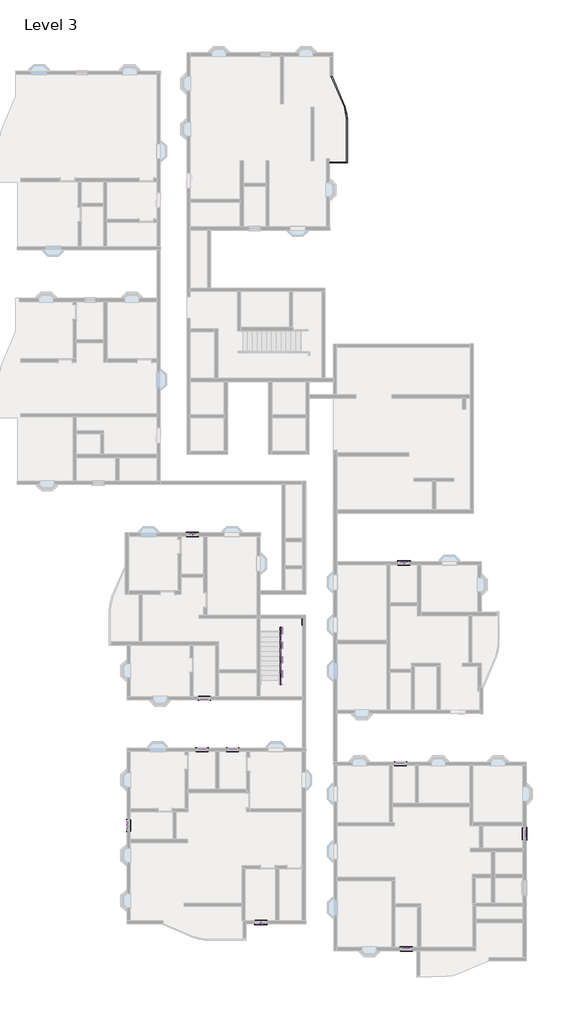
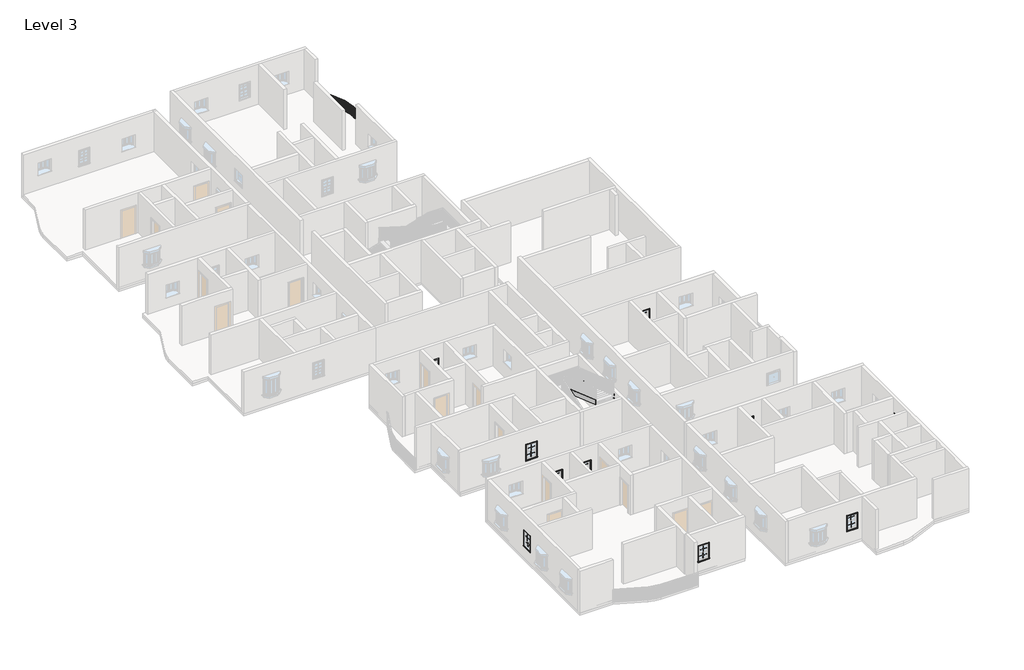
# One storey, part 13 of 14: 40 proxies, 6 members, 1 railing.
"""IFC4 building model written with IfcOpenShell, lengths in millimetres."""

from ifc_helpers import new_model, si_unit, frame, origin, place, context, project, spatial, polyline, circle_curve, outline, extrude, transform, mapped, element, save
from ifc_brep_helpers import plane_surface, cylinder_surface, revolved_surface, advanced_brep
from components import muntin_pattern_2x2_muntin_pattern_2x2_c35c595f, trim_window_exterior_flat_with_sill_e38017c9, trim_window_interior_flat_picture_frame_d728ed12

model = new_model("IFC4")

# Units and contexts
model_context = context("Model", 3, world=origin())
ifc_project = project(units=[si_unit("LENGTHUNIT", "METRE", prefix="MILLI")], contexts=[model_context])

# Site, building, storey
site = spatial("IfcSite", under=ifc_project)
building = spatial("IfcBuilding", under=site)
storey = spatial("IfcBuildingStorey", under=building, Name="Level 3", Elevation=6096.0)

# Proxies
placement = place(None, origin())
muntin_pattern_2x2_muntin_pattern_2x2_shape = muntin_pattern_2x2_muntin_pattern_2x2_c35c595f(model_context)
element("IfcBuildingElementProxy", 1, Name="Muntin Pattern_2x2 : Muntin Pattern_2x2", ObjectType="Muntin Pattern_2x2 : Muntin Pattern_2x2", at=placement, inside=storey, context=model_context, shape_type="MappedRepresentation", body=[
    mapped(muntin_pattern_2x2_muntin_pattern_2x2_shape, transform((-8150.287215, -357.5666506, 7566.025), x_axis=(1.0, 0.0, 0.0), y_axis=(0.0, 1.0, 0.0), z_axis=(0.0, 0.0, 1.0))),
])
element("IfcBuildingElementProxy", 2, Name="Muntin Pattern_2x2 : Muntin Pattern_2x2", ObjectType="Muntin Pattern_2x2 : Muntin Pattern_2x2", at=placement, inside=storey, context=model_context, shape_type="MappedRepresentation", body=[
    mapped(muntin_pattern_2x2_muntin_pattern_2x2_shape, transform((-8150.287215, -402.0166506, 7086.6), x_axis=(1.0, 0.0, 0.0), y_axis=(0.0, 1.0, 0.0), z_axis=(0.0, 0.0, 1.0))),
])
element("IfcBuildingElementProxy", 3, Name="Muntin Pattern_2x2 : Muntin Pattern_2x2", ObjectType="Muntin Pattern_2x2 : Muntin Pattern_2x2", at=placement, inside=storey, context=model_context, shape_type="MappedRepresentation", body=[
    mapped(muntin_pattern_2x2_muntin_pattern_2x2_shape, transform((-7397.812215, -10854.1166506, 7566.025), x_axis=(-1.0, 0.0, 0.0), y_axis=(0.0, -1.0, 0.0), z_axis=(0.0, 0.0, 1.0))),
])
element("IfcBuildingElementProxy", 4, Name="Muntin Pattern_2x2 : Muntin Pattern_2x2", ObjectType="Muntin Pattern_2x2 : Muntin Pattern_2x2", at=placement, inside=storey, context=model_context, shape_type="MappedRepresentation", body=[
    mapped(muntin_pattern_2x2_muntin_pattern_2x2_shape, transform((-7397.812215, -10809.6666506, 7086.6), x_axis=(-1.0, 0.0, 0.0), y_axis=(0.0, -1.0, 0.0), z_axis=(0.0, 0.0, 1.0))),
])
element("IfcBuildingElementProxy", 5, Name="Muntin Pattern_2x2 : Muntin Pattern_2x2", ObjectType="Muntin Pattern_2x2 : Muntin Pattern_2x2", at=placement, inside=storey, context=model_context, shape_type="MappedRepresentation", body=[
    mapped(muntin_pattern_2x2_muntin_pattern_2x2_shape, transform((-7540.687215, -13997.3666506, 7566.025), x_axis=(1.0, 0.0, 0.0), y_axis=(0.0, 1.0, 0.0), z_axis=(0.0, 0.0, 1.0))),
])
element("IfcBuildingElementProxy", 6, Name="Muntin Pattern_2x2 : Muntin Pattern_2x2", ObjectType="Muntin Pattern_2x2 : Muntin Pattern_2x2", at=placement, inside=storey, context=model_context, shape_type="MappedRepresentation", body=[
    mapped(muntin_pattern_2x2_muntin_pattern_2x2_shape, transform((-7540.687215, -14041.8166506, 7086.6), x_axis=(1.0, 0.0, 0.0), y_axis=(0.0, 1.0, 0.0), z_axis=(0.0, 0.0, 1.0))),
])
element("IfcBuildingElementProxy", 7, Name="Muntin Pattern_2x2 : Muntin Pattern_2x2", ObjectType="Muntin Pattern_2x2 : Muntin Pattern_2x2", at=placement, inside=storey, context=model_context, shape_type="MappedRepresentation", body=[
    mapped(muntin_pattern_2x2_muntin_pattern_2x2_shape, transform((-5597.587215, -13997.3666506, 7566.025), x_axis=(1.0, 0.0, 0.0), y_axis=(0.0, 1.0, 0.0), z_axis=(0.0, 0.0, 1.0))),
])
element("IfcBuildingElementProxy", 8, Name="Muntin Pattern_2x2 : Muntin Pattern_2x2", ObjectType="Muntin Pattern_2x2 : Muntin Pattern_2x2", at=placement, inside=storey, context=model_context, shape_type="MappedRepresentation", body=[
    mapped(muntin_pattern_2x2_muntin_pattern_2x2_shape, transform((-5597.587215, -14041.8166506, 7086.6), x_axis=(1.0, 0.0, 0.0), y_axis=(0.0, 1.0, 0.0), z_axis=(0.0, 0.0, 1.0))),
])
element("IfcBuildingElementProxy", 9, Name="Muntin Pattern_2x2 : Muntin Pattern_2x2", ObjectType="Muntin Pattern_2x2 : Muntin Pattern_2x2", at=placement, inside=storey, context=model_context, shape_type="MappedRepresentation", body=[
    mapped(muntin_pattern_2x2_muntin_pattern_2x2_shape, transform((-12255.562215, -18863.6994419, 7566.025), x_axis=(0.0, 1.0, 0.0), y_axis=(-1.0, 0.0, 0.0), z_axis=(0.0, 0.0, 1.0))),
])
element("IfcBuildingElementProxy", 10, Name="Muntin Pattern_2x2 : Muntin Pattern_2x2", ObjectType="Muntin Pattern_2x2 : Muntin Pattern_2x2", at=placement, inside=storey, context=model_context, shape_type="MappedRepresentation", body=[
    mapped(muntin_pattern_2x2_muntin_pattern_2x2_shape, transform((-12211.112215, -18863.6994419, 7086.6), x_axis=(0.0, 1.0, 0.0), y_axis=(-1.0, 0.0, 0.0), z_axis=(0.0, 0.0, 1.0))),
])
element("IfcBuildingElementProxy", 11, Name="Muntin Pattern_2x2 : Muntin Pattern_2x2", ObjectType="Muntin Pattern_2x2 : Muntin Pattern_2x2", at=placement, inside=storey, context=model_context, shape_type="MappedRepresentation", body=[
    mapped(muntin_pattern_2x2_muntin_pattern_2x2_shape, transform((-3806.2891351, -25065.4166506, 7566.025), x_axis=(-1.0, 0.0, 0.0), y_axis=(0.0, -1.0, 0.0), z_axis=(0.0, 0.0, 1.0))),
])
element("IfcBuildingElementProxy", 12, Name="Muntin Pattern_2x2 : Muntin Pattern_2x2", ObjectType="Muntin Pattern_2x2 : Muntin Pattern_2x2", at=placement, inside=storey, context=model_context, shape_type="MappedRepresentation", body=[
    mapped(muntin_pattern_2x2_muntin_pattern_2x2_shape, transform((-3806.2891351, -25020.9666506, 7086.6), x_axis=(-1.0, 0.0, 0.0), y_axis=(0.0, -1.0, 0.0), z_axis=(0.0, 0.0, 1.0))),
])
element("IfcBuildingElementProxy", 13, Name="Muntin Pattern_2x2 : Muntin Pattern_2x2", ObjectType="Muntin Pattern_2x2 : Muntin Pattern_2x2", at=placement, inside=storey, context=model_context, shape_type="MappedRepresentation", body=[
    mapped(muntin_pattern_2x2_muntin_pattern_2x2_shape, transform((5410.0380523, -26615.6292694, 7566.025), x_axis=(1.0, 0.0, 0.0), y_axis=(0.0, 1.0, 0.0), z_axis=(0.0, 0.0, 1.0))),
])
element("IfcBuildingElementProxy", 14, Name="Muntin Pattern_2x2 : Muntin Pattern_2x2", ObjectType="Muntin Pattern_2x2 : Muntin Pattern_2x2", at=placement, inside=storey, context=model_context, shape_type="MappedRepresentation", body=[
    mapped(muntin_pattern_2x2_muntin_pattern_2x2_shape, transform((5410.0380523, -26660.0792694, 7086.6), x_axis=(1.0, 0.0, 0.0), y_axis=(0.0, 1.0, 0.0), z_axis=(0.0, 0.0, 1.0))),
])
element("IfcBuildingElementProxy", 15, Name="Muntin Pattern_2x2 : Muntin Pattern_2x2", ObjectType="Muntin Pattern_2x2 : Muntin Pattern_2x2", at=placement, inside=storey, context=model_context, shape_type="MappedRepresentation", body=[
    mapped(muntin_pattern_2x2_muntin_pattern_2x2_shape, transform((12982.4130523, -19379.8042694, 7566.025), x_axis=(0.0, -1.0, 0.0), y_axis=(1.0, 0.0, 0.0), z_axis=(0.0, 0.0, 1.0))),
])
element("IfcBuildingElementProxy", 16, Name="Muntin Pattern_2x2 : Muntin Pattern_2x2", ObjectType="Muntin Pattern_2x2 : Muntin Pattern_2x2", at=placement, inside=storey, context=model_context, shape_type="MappedRepresentation", body=[
    mapped(muntin_pattern_2x2_muntin_pattern_2x2_shape, transform((12937.9630523, -19379.8042694, 7086.6), x_axis=(0.0, -1.0, 0.0), y_axis=(1.0, 0.0, 0.0), z_axis=(0.0, 0.0, 1.0))),
])
element("IfcBuildingElementProxy", 17, Name="Muntin Pattern_2x2 : Muntin Pattern_2x2", ObjectType="Muntin Pattern_2x2 : Muntin Pattern_2x2", at=placement, inside=storey, context=model_context, shape_type="MappedRepresentation", body=[
    mapped(muntin_pattern_2x2_muntin_pattern_2x2_shape, transform((5048.0880523, -14880.8292694, 7566.025), x_axis=(1.0, 0.0, 0.0), y_axis=(0.0, 1.0, 0.0), z_axis=(0.0, 0.0, 1.0))),
])
element("IfcBuildingElementProxy", 18, Name="Muntin Pattern_2x2 : Muntin Pattern_2x2", ObjectType="Muntin Pattern_2x2 : Muntin Pattern_2x2", at=placement, inside=storey, context=model_context, shape_type="MappedRepresentation", body=[
    mapped(muntin_pattern_2x2_muntin_pattern_2x2_shape, transform((5048.0880523, -14925.2792694, 7086.6), x_axis=(1.0, 0.0, 0.0), y_axis=(0.0, 1.0, 0.0), z_axis=(0.0, 0.0, 1.0))),
])
element("IfcBuildingElementProxy", 19, Name="Muntin Pattern_2x2 : Muntin Pattern_2x2", ObjectType="Muntin Pattern_2x2 : Muntin Pattern_2x2", at=placement, inside=storey, context=model_context, shape_type="MappedRepresentation", body=[
    mapped(muntin_pattern_2x2_muntin_pattern_2x2_shape, transform((5257.6380523, -2168.1292694, 7566.025), x_axis=(1.0, 0.0, 0.0), y_axis=(0.0, 1.0, 0.0), z_axis=(0.0, 0.0, 1.0))),
])
element("IfcBuildingElementProxy", 20, Name="Muntin Pattern_2x2 : Muntin Pattern_2x2", ObjectType="Muntin Pattern_2x2 : Muntin Pattern_2x2", at=placement, inside=storey, context=model_context, shape_type="MappedRepresentation", body=[
    mapped(muntin_pattern_2x2_muntin_pattern_2x2_shape, transform((5257.6380523, -2212.5792694, 7086.6), x_axis=(1.0, 0.0, 0.0), y_axis=(0.0, 1.0, 0.0), z_axis=(0.0, 0.0, 1.0))),
])
trim_window_exterior_flat_with_sill_shape = trim_window_exterior_flat_with_sill_e38017c9(model_context)
element("IfcBuildingElementProxy", 21, Name="Trim-Window-Exterior-Flat : with Sill", ObjectType="Trim-Window-Exterior-Flat : with Sill", at=placement, inside=storey, context=model_context, shape_type="MappedRepresentation", body=[
    mapped(trim_window_exterior_flat_with_sill_shape, transform((-8150.287215, -322.6416506, 8077.2), x_axis=(-1.0, 0.0, 0.0), y_axis=(0.0, 0.0, 1.0), z_axis=(0.0, 1.0, 0.0))),
])
element("IfcBuildingElementProxy", 22, Name="Trim-Window-Exterior-Flat : with Sill", ObjectType="Trim-Window-Exterior-Flat : with Sill", at=placement, inside=storey, context=model_context, shape_type="MappedRepresentation", body=[
    mapped(trim_window_exterior_flat_with_sill_shape, transform((-7397.812215, -10889.0416506, 8077.2), x_axis=(1.0, 0.0, 0.0), y_axis=(0.0, 0.0, 1.0), z_axis=(0.0, -1.0, 0.0))),
])
element("IfcBuildingElementProxy", 23, Name="Trim-Window-Exterior-Flat : with Sill", ObjectType="Trim-Window-Exterior-Flat : with Sill", at=placement, inside=storey, context=model_context, shape_type="MappedRepresentation", body=[
    mapped(trim_window_exterior_flat_with_sill_shape, transform((-7540.687215, -13962.4416506, 8077.2), x_axis=(-1.0, 0.0, 0.0), y_axis=(0.0, 0.0, 1.0), z_axis=(0.0, 1.0, 0.0))),
])
element("IfcBuildingElementProxy", 24, Name="Trim-Window-Exterior-Flat : with Sill", ObjectType="Trim-Window-Exterior-Flat : with Sill", at=placement, inside=storey, context=model_context, shape_type="MappedRepresentation", body=[
    mapped(trim_window_exterior_flat_with_sill_shape, transform((-5597.587215, -13962.4416506, 8077.2), x_axis=(-1.0, 0.0, 0.0), y_axis=(0.0, 0.0, 1.0), z_axis=(0.0, 1.0, 0.0))),
])
element("IfcBuildingElementProxy", 25, Name="Trim-Window-Exterior-Flat : with Sill", ObjectType="Trim-Window-Exterior-Flat : with Sill", at=placement, inside=storey, context=model_context, shape_type="MappedRepresentation", body=[
    mapped(trim_window_exterior_flat_with_sill_shape, transform((-12290.487215, -18863.6994419, 8077.2), x_axis=(0.0, -1.0, 0.0), y_axis=(0.0, 0.0, 1.0), z_axis=(-1.0, 0.0, 0.0))),
])
element("IfcBuildingElementProxy", 26, Name="Trim-Window-Exterior-Flat : with Sill", ObjectType="Trim-Window-Exterior-Flat : with Sill", at=placement, inside=storey, context=model_context, shape_type="MappedRepresentation", body=[
    mapped(trim_window_exterior_flat_with_sill_shape, transform((-3806.2891351, -25100.3416506, 8077.2), x_axis=(1.0, 0.0, 0.0), y_axis=(0.0, 0.0, 1.0), z_axis=(0.0, -1.0, 0.0))),
])
element("IfcBuildingElementProxy", 27, Name="Trim-Window-Exterior-Flat : with Sill", ObjectType="Trim-Window-Exterior-Flat : with Sill", at=placement, inside=storey, context=model_context, shape_type="MappedRepresentation", body=[
    mapped(trim_window_exterior_flat_with_sill_shape, transform((5410.0380523, -26580.7042694, 8077.2), x_axis=(-1.0, 0.0, 0.0), y_axis=(0.0, 0.0, 1.0), z_axis=(0.0, 1.0, 0.0))),
])
element("IfcBuildingElementProxy", 28, Name="Trim-Window-Exterior-Flat : with Sill", ObjectType="Trim-Window-Exterior-Flat : with Sill", at=placement, inside=storey, context=model_context, shape_type="MappedRepresentation", body=[
    mapped(trim_window_exterior_flat_with_sill_shape, transform((13017.3380523, -19379.8042694, 8077.2), x_axis=(0.0, 1.0, 0.0), y_axis=(0.0, 0.0, 1.0), z_axis=(1.0, 0.0, 0.0))),
])
element("IfcBuildingElementProxy", 29, Name="Trim-Window-Exterior-Flat : with Sill", ObjectType="Trim-Window-Exterior-Flat : with Sill", at=placement, inside=storey, context=model_context, shape_type="MappedRepresentation", body=[
    mapped(trim_window_exterior_flat_with_sill_shape, transform((5048.0880523, -14845.9042694, 8077.2), x_axis=(-1.0, 0.0, 0.0), y_axis=(0.0, 0.0, 1.0), z_axis=(0.0, 1.0, 0.0))),
])
element("IfcBuildingElementProxy", 30, Name="Trim-Window-Exterior-Flat : with Sill", ObjectType="Trim-Window-Exterior-Flat : with Sill", at=placement, inside=storey, context=model_context, shape_type="MappedRepresentation", body=[
    mapped(trim_window_exterior_flat_with_sill_shape, transform((5257.6380523, -2133.2042694, 8077.2), x_axis=(-1.0, 0.0, 0.0), y_axis=(0.0, 0.0, 1.0), z_axis=(0.0, 1.0, 0.0))),
])
trim_window_interior_flat_picture_frame_shape = trim_window_interior_flat_picture_frame_d728ed12(model_context)
element("IfcBuildingElementProxy", 31, Name="Trim-Window-Interior-Flat : Picture Frame", ObjectType="Trim-Window-Interior-Flat : Picture Frame", at=placement, inside=storey, context=model_context, shape_type="MappedRepresentation", body=[
    mapped(trim_window_interior_flat_picture_frame_shape, transform((-8150.287215, -525.8416506, 8077.2), x_axis=(1.0, 0.0, 0.0), y_axis=(0.0, 0.0, 1.0), z_axis=(0.0, -1.0, 0.0))),
])
element("IfcBuildingElementProxy", 32, Name="Trim-Window-Interior-Flat : Picture Frame", ObjectType="Trim-Window-Interior-Flat : Picture Frame", at=placement, inside=storey, context=model_context, shape_type="MappedRepresentation", body=[
    mapped(trim_window_interior_flat_picture_frame_shape, transform((-7397.812215, -10685.8416506, 8077.2), x_axis=(-1.0, 0.0, 0.0), y_axis=(0.0, 0.0, 1.0), z_axis=(0.0, 1.0, 0.0))),
])
element("IfcBuildingElementProxy", 33, Name="Trim-Window-Interior-Flat : Picture Frame", ObjectType="Trim-Window-Interior-Flat : Picture Frame", at=placement, inside=storey, context=model_context, shape_type="MappedRepresentation", body=[
    mapped(trim_window_interior_flat_picture_frame_shape, transform((-7540.687215, -14165.6416506, 8077.2), x_axis=(1.0, 0.0, 0.0), y_axis=(0.0, 0.0, 1.0), z_axis=(0.0, -1.0, 0.0))),
])
element("IfcBuildingElementProxy", 34, Name="Trim-Window-Interior-Flat : Picture Frame", ObjectType="Trim-Window-Interior-Flat : Picture Frame", at=placement, inside=storey, context=model_context, shape_type="MappedRepresentation", body=[
    mapped(trim_window_interior_flat_picture_frame_shape, transform((-5597.587215, -14165.6416506, 8077.2), x_axis=(1.0, 0.0, 0.0), y_axis=(0.0, 0.0, 1.0), z_axis=(0.0, -1.0, 0.0))),
])
element("IfcBuildingElementProxy", 35, Name="Trim-Window-Interior-Flat : Picture Frame", ObjectType="Trim-Window-Interior-Flat : Picture Frame", at=placement, inside=storey, context=model_context, shape_type="MappedRepresentation", body=[
    mapped(trim_window_interior_flat_picture_frame_shape, transform((-12087.287215, -18863.6994419, 8077.2), x_axis=(0.0, 1.0, 0.0), y_axis=(0.0, 0.0, 1.0), z_axis=(1.0, 0.0, 0.0))),
])
element("IfcBuildingElementProxy", 36, Name="Trim-Window-Interior-Flat : Picture Frame", ObjectType="Trim-Window-Interior-Flat : Picture Frame", at=placement, inside=storey, context=model_context, shape_type="MappedRepresentation", body=[
    mapped(trim_window_interior_flat_picture_frame_shape, transform((-3806.2891351, -24897.1416506, 8077.2), x_axis=(-1.0, 0.0, 0.0), y_axis=(0.0, 0.0, 1.0), z_axis=(0.0, 1.0, 0.0))),
])
element("IfcBuildingElementProxy", 37, Name="Trim-Window-Interior-Flat : Picture Frame", ObjectType="Trim-Window-Interior-Flat : Picture Frame", at=placement, inside=storey, context=model_context, shape_type="MappedRepresentation", body=[
    mapped(trim_window_interior_flat_picture_frame_shape, transform((5410.0380523, -26783.9042694, 8077.2), x_axis=(1.0, 0.0, 0.0), y_axis=(0.0, 0.0, 1.0), z_axis=(0.0, -1.0, 0.0))),
])
element("IfcBuildingElementProxy", 38, Name="Trim-Window-Interior-Flat : Picture Frame", ObjectType="Trim-Window-Interior-Flat : Picture Frame", at=placement, inside=storey, context=model_context, shape_type="MappedRepresentation", body=[
    mapped(trim_window_interior_flat_picture_frame_shape, transform((12814.1380523, -19379.8042694, 8077.2), x_axis=(0.0, -1.0, 0.0), y_axis=(0.0, 0.0, 1.0), z_axis=(-1.0, 0.0, 0.0))),
])
element("IfcBuildingElementProxy", 39, Name="Trim-Window-Interior-Flat : Picture Frame", ObjectType="Trim-Window-Interior-Flat : Picture Frame", at=placement, inside=storey, context=model_context, shape_type="MappedRepresentation", body=[
    mapped(trim_window_interior_flat_picture_frame_shape, transform((5048.0880523, -15049.1042694, 8077.2), x_axis=(1.0, 0.0, 0.0), y_axis=(0.0, 0.0, 1.0), z_axis=(0.0, -1.0, 0.0))),
])
element("IfcBuildingElementProxy", 40, Name="Trim-Window-Interior-Flat : Picture Frame", ObjectType="Trim-Window-Interior-Flat : Picture Frame", at=placement, inside=storey, context=model_context, shape_type="MappedRepresentation", body=[
    mapped(trim_window_interior_flat_picture_frame_shape, transform((5257.6380523, -2336.4042694, 8077.2), x_axis=(1.0, 0.0, 0.0), y_axis=(0.0, 0.0, 1.0), z_axis=(0.0, -1.0, 0.0))),
])

# Members
element("IfcMember", 41, ObjectType="Stringer - 2\" Width", at=placement, inside=storey, context=model_context, shape_type="SweptSolid", body=[
    extrude(outline(polyline([(-9955.5916506, 6096.0), (-9955.5916506, 6287.3592169), (-6325.8738327, 7543.8), (-5713.7916506, 7543.8), (-5713.7916506, 7433.1301656), (-9576.612129, 6096.0), (-9955.5916506, 6096.0)])), frame((-3908.487215, 0.0, 0.0), z_axis=(1.0, 0.0, 0.0), x_axis=(0.0, 1.0, 0.0)), (0.0, 0.0, 1.0), 50.8),
])
element("IfcMember", 42, ObjectType="Stringer - 2\" Width", at=placement, inside=storey, context=model_context, shape_type="SweptSolid", body=[
    extrude(outline(polyline([(-3908.487215, -5713.7916506), (-3908.487215, -5662.9916506), (-1190.687215, -5662.9916506), (-1190.687215, -5713.7916506), (-3908.487215, -5713.7916506)])), frame((0.0, 0.0, 7239.0), z_axis=(0.0, 0.0, 1.0), x_axis=(1.0, 0.0, 0.0)), (0.0, 0.0, 1.0), 304.8),
])
element("IfcMember", 43, ObjectType="Stringer - 2\" Width", at=placement, inside=storey, context=model_context, shape_type="SweptSolid", body=[
    extrude(outline(polyline([(-5662.9916506, 7443.5476784), (-5662.9916506, 7239.0), (-6003.8711722, 7239.0), (-9949.2416506, 8604.7051656), (-9949.2416506, 8927.2496015), (-5662.9916506, 7443.5476784)])), frame((-1190.687215, 0.0, 0.0), z_axis=(1.0, 0.0, 0.0), x_axis=(0.0, 1.0, 0.0)), (0.0, 0.0, 1.0), 50.8),
])
element("IfcMember", 44, ObjectType="Stringer - 2\" Width", at=placement, inside=storey, context=model_context, shape_type="SweptSolid", body=[
    extrude(outline(polyline([(-9955.5916506, 6096.0), (-9955.5916506, 6287.3592169), (-6342.4416506, 7538.0649861), (-6342.4416506, 7215.5205502), (-9576.612129, 6096.0), (-9955.5916506, 6096.0)])), frame((-2593.7381751, 0.0, 0.0), z_axis=(1.0, 0.0, 0.0), x_axis=(0.0, 1.0, 0.0)), (0.0, 0.0, 1.0), 50.8),
])
element("IfcMember", 45, ObjectType="Stringer - 2\" Width", at=placement, inside=storey, context=model_context, shape_type="SweptSolid", body=[
    extrude(outline(polyline([(-2593.7381751, -6342.4416506), (-2593.7381751, -6291.6416506), (-2492.1381751, -6291.6416506), (-2492.1381751, -6342.4416506), (-2593.7381751, -6342.4416506)])), frame((0.0, 0.0, 7239.0), z_axis=(0.0, 0.0, 1.0), x_axis=(1.0, 0.0, 0.0)), (0.0, 0.0, 1.0), 304.8),
])
element("IfcMember", 46, ObjectType="Stringer - 2\" Width", at=placement, inside=storey, context=model_context, shape_type="SweptSolid", body=[
    extrude(outline(polyline([(-6291.6416506, 7661.1572938), (-6291.6416506, 7338.6128579), (-9949.2416506, 8604.7051656), (-9949.2416506, 8927.2496015), (-6291.6416506, 7661.1572938)])), frame((-2492.1381751, 0.0, 0.0), z_axis=(1.0, 0.0, 0.0), x_axis=(0.0, 1.0, 0.0)), (0.0, 0.0, 1.0), 50.8),
])

# Railing
element("IfcRailing", 47, ObjectType="Handrail - Rectangular", at=placement, inside=storey, context=model_context, shape_type="SolidModel", body=[
    advanced_brep(
    [(549.8108649, 23180.4215905, 7010.4), (549.8108649, 23180.4215905, 6959.6), (549.8108649, 23129.6215905, 6959.6), (549.8108649, 23129.6215905, 7010.4), (1629.3108649, 23180.4215905, 7010.4), (1629.3108649, 23180.4215905, 6959.6), (1680.1108649, 23129.6215905, 6959.6), (1680.1108649, 23129.6215905, 7010.4), (1629.3108649, 25921.9580583, 7010.4), (1629.3108649, 25921.9580583, 6959.6), (1680.1108649, 25921.9580583, 6959.6), (1680.1108649, 25921.9580583, 7010.4), (1475.5051478, 26671.8537734, 6959.6), (1475.5051478, 26671.8537734, 7010.4), (1522.203662, 26691.8509925, 6959.6), (1522.203662, 26691.8509925, 7010.4), (640.7616078, 28621.188975, 7010.4), (687.460122, 28641.186194, 7010.4), (687.460122, 28641.186194, 6959.6), (640.7616078, 28621.188975, 6959.6)],
    [
        (0, 1),
        (1, 2),
        (2, 3),
        (3, 0),
        (0, 4),
        (4, 5),
        (5, 1),
        (5, 6),
        (6, 2),
        (6, 7),
        (7, 3),
        (7, 4),
        (4, 8),
        (8, 9),
        (9, 5),
        (9, 10),
        (10, 6),
        (10, 11),
        (11, 7),
        (11, 8),
        (12, 9, circle_curve(frame((-275.6891351, 25921.9580583, 6959.6), z_axis=(0.0, 0.0, -1.0), x_axis=(1.0, 0.0, 0.0)), 1905.0)),
        (8, 13, circle_curve(frame((-275.6891351, 25921.9580583, 7010.4), z_axis=(0.0, 0.0, 1.0), x_axis=(1.0, 0.0, 0.0)), 1905.0)),
        (13, 12),
        (14, 10, circle_curve(frame((-275.6891351, 25921.9580583, 6959.6), z_axis=(0.0, 0.0, -1.0), x_axis=(1.0, 0.0, 0.0)), 1955.8)),
        (12, 14),
        (15, 11, circle_curve(frame((-275.6891351, 25921.9580583, 7010.4), z_axis=(0.0, 0.0, -1.0), x_axis=(1.0, 0.0, 0.0)), 1955.8)),
        (14, 15),
        (15, 13),
        (16, 17),
        (17, 18),
        (18, 19),
        (19, 16),
        (13, 16),
        (19, 12),
        (18, 14),
        (17, 15),
    ],
    [
        plane_surface(frame((549.8108649, 23155.0215905, 7010.4), z_axis=(-1.0, 0.0, 0.0), x_axis=(0.0, 1.0, 0.0))),
        plane_surface(frame((549.8108649, 23180.4215905, 7010.4), z_axis=(0.0, 1.0, 0.0), x_axis=(1.0, 0.0, 0.0))),
        plane_surface(frame((549.8108649, 23180.4215905, 6959.6), z_axis=(0.0, 0.0, -1.0), x_axis=(1.0, 0.0, 0.0))),
        plane_surface(frame((549.8108649, 23129.6215905, 6959.6), z_axis=(0.0, -1.0, 0.0), x_axis=(1.0, 0.0, 0.0))),
        plane_surface(frame((549.8108649, 23129.6215905, 7010.4), z_axis=(0.0, 0.0, 1.0), x_axis=(1.0, 0.0, 0.0))),
        plane_surface(frame((1629.3108649, 23180.4215905, 7010.4), z_axis=(-1.0, 0.0, 0.0), x_axis=(0.0, 1.0, 0.0))),
        plane_surface(frame((1629.3108649, 23180.4215905, 6959.6), z_axis=(0.0, 0.0, -1.0), x_axis=(0.0, 1.0, 0.0))),
        plane_surface(frame((1680.1108649, 23129.6215905, 6959.6), z_axis=(1.0, 0.0, 0.0), x_axis=(0.0, 1.0, 0.0))),
        plane_surface(frame((1680.1108649, 23129.6215905, 7010.4), z_axis=(0.0, 0.0, 1.0), x_axis=(0.0, 1.0, 0.0))),
        revolved_surface(polyline([(1629.3108649, 25921.9580583, 7010.4), (1629.3108649, 25921.9580583, 6959.6)]), (-275.6891351, 25921.9580583, 7010.4), (0.0, 0.0, 1.0)),
        plane_surface(frame((-275.6891351, 25921.9580583, 6959.6), z_axis=(0.0, 0.0, -1.0), x_axis=(1.0, 0.0, 0.0))),
        cylinder_surface(frame((-275.6891351, 25921.9580583, 7010.4), z_axis=(0.0, 0.0, 1.0), x_axis=(1.0, 0.0, 0.0)), 1955.8),
        plane_surface(frame((-275.6891351, 25921.9580583, 7010.4), z_axis=(0.0, 0.0, 1.0), x_axis=(1.0, 0.0, 0.0))),
        plane_surface(frame((664.1108649, 28631.1875845, 7010.4), z_axis=(-0.39364604467361036, 0.91926209076238, 0.0), x_axis=(0.91926209076238, 0.39364604467361036, 0.0))),
        plane_surface(frame((1475.5051478, 26671.8537734, 7010.4), z_axis=(-0.9192620907623801, -0.39364604467361014, 0.0), x_axis=(-0.39364604467361014, 0.9192620907623801, 0.0))),
        plane_surface(frame((1475.5051478, 26671.8537734, 6959.6), z_axis=(0.0, 0.0, -1.0000000000000002), x_axis=(-0.39364604467361014, 0.9192620907623801, 0.0))),
        plane_surface(frame((1522.203662, 26691.8509925, 6959.6), z_axis=(0.91926209076238, 0.3936460446736102, 0.0), x_axis=(-0.3936460446736102, 0.91926209076238, 0.0))),
        plane_surface(frame((1522.203662, 26691.8509925, 7010.4), z_axis=(0.0, 0.0, 1.0), x_axis=(-0.3936460446736102, 0.91926209076238, 0.0))),
    ],
    [
        (0, [[1, 2, 3, 4]]),
        (1, [[-1, 5, 6, 7]]),
        (2, [[-2, -7, 8, 9]]),
        (3, [[-3, -9, 10, 11]]),
        (4, [[-4, -11, 12, -5]]),
        (5, [[-6, 13, 14, 15]]),
        (6, [[-8, -15, 16, 17]]),
        (7, [[-10, -17, 18, 19]]),
        (8, [[-12, -19, 20, -13]]),
        (9, [[21, -14, 22, 23]]),
        (10, [[24, -16, -21, 25]]),
        (11, [[26, -18, -24, 27]]),
        (12, [[-22, -20, -26, 28]]),
        (13, [[29, 30, 31, 32]]),
        (14, [[-23, 33, -32, 34]]),
        (15, [[-25, -34, -31, 35]]),
        (16, [[-27, -35, -30, 36]]),
        (17, [[-28, -36, -29, -33]]),
    ],
),
    extrude(outline(polyline([(711.4710921, 28544.7864585), (693.9591493, 28537.2875014), (686.4601921, 28554.7994442), (703.9721349, 28562.2984014), (711.4710921, 28544.7864585)])), frame((0.0, 0.0, 6096.0), z_axis=(0.0, 0.0, 1.0), x_axis=(1.0, 0.0, 0.0)), (0.0, 0.0, 1.0), 863.6),
    extrude(outline(polyline([(751.4655302, 28451.3894301), (733.9535874, 28443.890473), (726.4546303, 28461.4024158), (743.9665731, 28468.9013729), (751.4655302, 28451.3894301)])), frame((0.0, 0.0, 6096.0), z_axis=(0.0, 0.0, 1.0), x_axis=(1.0, 0.0, 0.0)), (0.0, 0.0, 1.0), 863.6),
    extrude(outline(polyline([(791.4599684, 28357.9924017), (773.9480255, 28350.4934445), (766.4490684, 28368.0053874), (783.9610112, 28375.5043445), (791.4599684, 28357.9924017)])), frame((0.0, 0.0, 6096.0), z_axis=(0.0, 0.0, 1.0), x_axis=(1.0, 0.0, 0.0)), (0.0, 0.0, 1.0), 863.6),
    extrude(outline(polyline([(831.4544065, 28264.5953733), (813.9424637, 28257.0964161), (806.4435065, 28274.608359), (823.9554494, 28282.1073161), (831.4544065, 28264.5953733)])), frame((0.0, 0.0, 6096.0), z_axis=(0.0, 0.0, 1.0), x_axis=(1.0, 0.0, 0.0)), (0.0, 0.0, 1.0), 863.6),
    extrude(outline(polyline([(871.4488446, 28171.1983449), (853.9369018, 28163.6993877), (846.4379447, 28181.2113305), (863.9498875, 28188.7102877), (871.4488446, 28171.1983449)])), frame((0.0, 0.0, 6096.0), z_axis=(0.0, 0.0, 1.0), x_axis=(1.0, 0.0, 0.0)), (0.0, 0.0, 1.0), 863.6),
    extrude(outline(polyline([(911.4432828, 28077.8013164), (893.93134, 28070.3023593), (886.4323828, 28087.8143021), (903.9443256, 28095.3132593), (911.4432828, 28077.8013164)])), frame((0.0, 0.0, 6096.0), z_axis=(0.0, 0.0, 1.0), x_axis=(1.0, 0.0, 0.0)), (0.0, 0.0, 1.0), 863.6),
    extrude(outline(polyline([(951.4377209, 27984.404288), (933.9257781, 27976.9053309), (926.4268209, 27994.4172737), (943.9387638, 28001.9162308), (951.4377209, 27984.404288)])), frame((0.0, 0.0, 6096.0), z_axis=(0.0, 0.0, 1.0), x_axis=(1.0, 0.0, 0.0)), (0.0, 0.0, 1.0), 863.6),
    extrude(outline(polyline([(991.4321591, 27891.0072596), (973.9202162, 27883.5083024), (966.4212591, 27901.0202453), (983.9332019, 27908.5192024), (991.4321591, 27891.0072596)])), frame((0.0, 0.0, 6096.0), z_axis=(0.0, 0.0, 1.0), x_axis=(1.0, 0.0, 0.0)), (0.0, 0.0, 1.0), 863.6),
    extrude(outline(polyline([(1031.4265972, 27797.6102312), (1013.9146544, 27790.111274), (1006.4156972, 27807.6232168), (1023.9276401, 27815.122174), (1031.4265972, 27797.6102312)])), frame((0.0, 0.0, 6096.0), z_axis=(0.0, 0.0, 1.0), x_axis=(1.0, 0.0, 0.0)), (0.0, 0.0, 1.0), 863.6),
    extrude(outline(polyline([(1071.4210353, 27704.2132027), (1053.9090925, 27696.7142456), (1046.4101354, 27714.2261884), (1063.9220782, 27721.7251456), (1071.4210353, 27704.2132027)])), frame((0.0, 0.0, 6096.0), z_axis=(0.0, 0.0, 1.0), x_axis=(1.0, 0.0, 0.0)), (0.0, 0.0, 1.0), 863.6),
    extrude(outline(polyline([(1111.4154735, 27610.8161743), (1093.9035307, 27603.3172172), (1086.4045735, 27620.82916), (1103.9165163, 27628.3281172), (1111.4154735, 27610.8161743)])), frame((0.0, 0.0, 6096.0), z_axis=(0.0, 0.0, 1.0), x_axis=(1.0, 0.0, 0.0)), (0.0, 0.0, 1.0), 863.6),
    extrude(outline(polyline([(1151.4099116, 27517.4191459), (1133.8979688, 27509.9201888), (1126.3990116, 27527.4321316), (1143.9109545, 27534.9310887), (1151.4099116, 27517.4191459)])), frame((0.0, 0.0, 6096.0), z_axis=(0.0, 0.0, 1.0), x_axis=(1.0, 0.0, 0.0)), (0.0, 0.0, 1.0), 863.6),
    extrude(outline(polyline([(1191.4043498, 27424.0221175), (1173.8924069, 27416.5231603), (1166.3934498, 27434.0351032), (1183.9053926, 27441.5340603), (1191.4043498, 27424.0221175)])), frame((0.0, 0.0, 6096.0), z_axis=(0.0, 0.0, 1.0), x_axis=(1.0, 0.0, 0.0)), (0.0, 0.0, 1.0), 863.6),
    extrude(outline(polyline([(1231.3987879, 27330.6250891), (1213.8868451, 27323.1261319), (1206.3878879, 27340.6380747), (1223.8998307, 27348.1370319), (1231.3987879, 27330.6250891)])), frame((0.0, 0.0, 6096.0), z_axis=(0.0, 0.0, 1.0), x_axis=(1.0, 0.0, 0.0)), (0.0, 0.0, 1.0), 863.6),
    extrude(outline(polyline([(1271.393226, 27237.2280606), (1253.8812832, 27229.7291035), (1246.3823261, 27247.2410463), (1263.8942689, 27254.7400035), (1271.393226, 27237.2280606)])), frame((0.0, 0.0, 6096.0), z_axis=(0.0, 0.0, 1.0), x_axis=(1.0, 0.0, 0.0)), (0.0, 0.0, 1.0), 863.6),
    extrude(outline(polyline([(1311.3876642, 27143.8310322), (1293.8757213, 27136.3320751), (1286.3767642, 27153.8440179), (1303.888707, 27161.342975), (1311.3876642, 27143.8310322)])), frame((0.0, 0.0, 6096.0), z_axis=(0.0, 0.0, 1.0), x_axis=(1.0, 0.0, 0.0)), (0.0, 0.0, 1.0), 863.6),
    extrude(outline(polyline([(1351.3821023, 27050.4340038), (1333.8701595, 27042.9350466), (1326.3712023, 27060.4469895), (1343.8831452, 27067.9459466), (1351.3821023, 27050.4340038)])), frame((0.0, 0.0, 6096.0), z_axis=(0.0, 0.0, 1.0), x_axis=(1.0, 0.0, 0.0)), (0.0, 0.0, 1.0), 863.6),
    extrude(outline(polyline([(1391.3765405, 26957.0369754), (1373.8645976, 26949.5380182), (1366.3656405, 26967.0499611), (1383.8775833, 26974.5489182), (1391.3765405, 26957.0369754)])), frame((0.0, 0.0, 6096.0), z_axis=(0.0, 0.0, 1.0), x_axis=(1.0, 0.0, 0.0)), (0.0, 0.0, 1.0), 863.6),
    extrude(outline(polyline([(1431.3709786, 26863.639947), (1413.8590358, 26856.1409898), (1406.3600786, 26873.6529326), (1423.8720214, 26881.1518898), (1431.3709786, 26863.639947)])), frame((0.0, 0.0, 6096.0), z_axis=(0.0, 0.0, 1.0), x_axis=(1.0, 0.0, 0.0)), (0.0, 0.0, 1.0), 863.6),
    extrude(outline(polyline([(1471.3654167, 26770.2429185), (1453.8534739, 26762.7439614), (1446.3545168, 26780.2559042), (1463.8664596, 26787.7548614), (1471.3654167, 26770.2429185)])), frame((0.0, 0.0, 6096.0), z_axis=(0.0, 0.0, 1.0), x_axis=(1.0, 0.0, 0.0)), (0.0, 0.0, 1.0), 863.6),
    extrude(outline(polyline([(1537.4917391, 26611.722401), (1519.7200483, 26604.8616791), (1512.8593263, 26622.6333699), (1530.6310171, 26629.4940918), (1537.4917391, 26611.722401)])), frame((0.0, 0.0, 6096.0), z_axis=(0.0, 0.0, 1.0), x_axis=(1.0, 0.0, 0.0)), (0.0, 0.0, 1.0), 863.6),
    extrude(outline(polyline([(1571.2676162, 26515.3807493), (1553.1596103, 26509.4644479), (1547.2433088, 26527.5724538), (1565.3513147, 26533.4887552), (1571.2676162, 26515.3807493)])), frame((0.0, 0.0, 6096.0), z_axis=(0.0, 0.0, 1.0), x_axis=(1.0, 0.0, 0.0)), (0.0, 0.0, 1.0), 863.6),
    extrude(outline(polyline([(1599.9284504, 26417.3956468), (1581.5342785, 26412.4401508), (1576.5787825, 26430.8343227), (1594.9729544, 26435.7898187), (1599.9284504, 26417.3956468)])), frame((0.0, 0.0, 6096.0), z_axis=(0.0, 0.0, 1.0), x_axis=(1.0, 0.0, 0.0)), (0.0, 0.0, 1.0), 863.6),
    extrude(outline(polyline([(1623.3948673, 26318.0384578), (1604.7654711, 26314.0574912), (1600.7845045, 26332.6868874), (1619.4139008, 26336.667854), (1623.3948673, 26318.0384578)])), frame((0.0, 0.0, 6096.0), z_axis=(0.0, 0.0, 1.0), x_axis=(1.0, 0.0, 0.0)), (0.0, 0.0, 1.0), 863.6),
    extrude(outline(polyline([(1641.601878, 26217.5843464), (1622.7888504, 26214.5889343), (1619.7934383, 26233.4019618), (1638.6064659, 26236.3973739), (1641.601878, 26217.5843464)])), frame((0.0, 0.0, 6096.0), z_axis=(0.0, 0.0, 1.0), x_axis=(1.0, 0.0, 0.0)), (0.0, 0.0, 1.0), 863.6),
    extrude(outline(polyline([(1654.4990591, 26116.3115146), (1635.5545019, 26114.3099526), (1633.5529398, 26133.2545098), (1652.4974971, 26135.2560719), (1654.4990591, 26116.3115146)])), frame((0.0, 0.0, 6096.0), z_axis=(0.0, 0.0, 1.0), x_axis=(1.0, 0.0, 0.0)), (0.0, 0.0, 1.0), 863.6),
    extrude(outline(polyline([(1662.0506927, 26014.5004319), (1643.0270716, 26013.4982632), (1642.0249029, 26032.5218842), (1661.048524, 26033.524053), (1662.0506927, 26014.5004319)])), frame((0.0, 0.0, 6096.0), z_axis=(0.0, 0.0, 1.0), x_axis=(1.0, 0.0, 0.0)), (0.0, 0.0, 1.0), 863.6),
    extrude(outline(polyline([(1664.2358649, 25888.6965905), (1645.1858649, 25888.6965905), (1645.1858649, 25907.7465905), (1664.2358649, 25907.7465905), (1664.2358649, 25888.6965905)])), frame((0.0, 0.0, 6096.0), z_axis=(0.0, 0.0, 1.0), x_axis=(1.0, 0.0, 0.0)), (0.0, 0.0, 1.0), 863.6),
    extrude(outline(polyline([(1664.2358649, 25787.0965905), (1645.1858649, 25787.0965905), (1645.1858649, 25806.1465905), (1664.2358649, 25806.1465905), (1664.2358649, 25787.0965905)])), frame((0.0, 0.0, 6096.0), z_axis=(0.0, 0.0, 1.0), x_axis=(1.0, 0.0, 0.0)), (0.0, 0.0, 1.0), 863.6),
    extrude(outline(polyline([(1664.2358649, 25685.4965905), (1645.1858649, 25685.4965905), (1645.1858649, 25704.5465905), (1664.2358649, 25704.5465905), (1664.2358649, 25685.4965905)])), frame((0.0, 0.0, 6096.0), z_axis=(0.0, 0.0, 1.0), x_axis=(1.0, 0.0, 0.0)), (0.0, 0.0, 1.0), 863.6),
    extrude(outline(polyline([(1664.2358649, 25583.8965905), (1645.1858649, 25583.8965905), (1645.1858649, 25602.9465905), (1664.2358649, 25602.9465905), (1664.2358649, 25583.8965905)])), frame((0.0, 0.0, 6096.0), z_axis=(0.0, 0.0, 1.0), x_axis=(1.0, 0.0, 0.0)), (0.0, 0.0, 1.0), 863.6),
    extrude(outline(polyline([(1664.2358649, 25482.2965905), (1645.1858649, 25482.2965905), (1645.1858649, 25501.3465905), (1664.2358649, 25501.3465905), (1664.2358649, 25482.2965905)])), frame((0.0, 0.0, 6096.0), z_axis=(0.0, 0.0, 1.0), x_axis=(1.0, 0.0, 0.0)), (0.0, 0.0, 1.0), 863.6),
    extrude(outline(polyline([(1664.2358649, 25380.6965905), (1645.1858649, 25380.6965905), (1645.1858649, 25399.7465905), (1664.2358649, 25399.7465905), (1664.2358649, 25380.6965905)])), frame((0.0, 0.0, 6096.0), z_axis=(0.0, 0.0, 1.0), x_axis=(1.0, 0.0, 0.0)), (0.0, 0.0, 1.0), 863.6),
    extrude(outline(polyline([(1664.2358649, 25279.0965905), (1645.1858649, 25279.0965905), (1645.1858649, 25298.1465905), (1664.2358649, 25298.1465905), (1664.2358649, 25279.0965905)])), frame((0.0, 0.0, 6096.0), z_axis=(0.0, 0.0, 1.0), x_axis=(1.0, 0.0, 0.0)), (0.0, 0.0, 1.0), 863.6),
    extrude(outline(polyline([(1664.2358649, 25177.4965905), (1645.1858649, 25177.4965905), (1645.1858649, 25196.5465905), (1664.2358649, 25196.5465905), (1664.2358649, 25177.4965905)])), frame((0.0, 0.0, 6096.0), z_axis=(0.0, 0.0, 1.0), x_axis=(1.0, 0.0, 0.0)), (0.0, 0.0, 1.0), 863.6),
    extrude(outline(polyline([(1664.2358649, 25075.8965905), (1645.1858649, 25075.8965905), (1645.1858649, 25094.9465905), (1664.2358649, 25094.9465905), (1664.2358649, 25075.8965905)])), frame((0.0, 0.0, 6096.0), z_axis=(0.0, 0.0, 1.0), x_axis=(1.0, 0.0, 0.0)), (0.0, 0.0, 1.0), 863.6),
    extrude(outline(polyline([(1664.2358649, 24974.2965905), (1645.1858649, 24974.2965905), (1645.1858649, 24993.3465905), (1664.2358649, 24993.3465905), (1664.2358649, 24974.2965905)])), frame((0.0, 0.0, 6096.0), z_axis=(0.0, 0.0, 1.0), x_axis=(1.0, 0.0, 0.0)), (0.0, 0.0, 1.0), 863.6),
    extrude(outline(polyline([(1664.2358649, 24872.6965905), (1645.1858649, 24872.6965905), (1645.1858649, 24891.7465905), (1664.2358649, 24891.7465905), (1664.2358649, 24872.6965905)])), frame((0.0, 0.0, 6096.0), z_axis=(0.0, 0.0, 1.0), x_axis=(1.0, 0.0, 0.0)), (0.0, 0.0, 1.0), 863.6),
    extrude(outline(polyline([(1664.2358649, 24771.0965905), (1645.1858649, 24771.0965905), (1645.1858649, 24790.1465905), (1664.2358649, 24790.1465905), (1664.2358649, 24771.0965905)])), frame((0.0, 0.0, 6096.0), z_axis=(0.0, 0.0, 1.0), x_axis=(1.0, 0.0, 0.0)), (0.0, 0.0, 1.0), 863.6),
    extrude(outline(polyline([(1664.2358649, 24669.4965905), (1645.1858649, 24669.4965905), (1645.1858649, 24688.5465905), (1664.2358649, 24688.5465905), (1664.2358649, 24669.4965905)])), frame((0.0, 0.0, 6096.0), z_axis=(0.0, 0.0, 1.0), x_axis=(1.0, 0.0, 0.0)), (0.0, 0.0, 1.0), 863.6),
    extrude(outline(polyline([(1664.2358649, 24567.8965905), (1645.1858649, 24567.8965905), (1645.1858649, 24586.9465905), (1664.2358649, 24586.9465905), (1664.2358649, 24567.8965905)])), frame((0.0, 0.0, 6096.0), z_axis=(0.0, 0.0, 1.0), x_axis=(1.0, 0.0, 0.0)), (0.0, 0.0, 1.0), 863.6),
    extrude(outline(polyline([(1664.2358649, 24466.2965905), (1645.1858649, 24466.2965905), (1645.1858649, 24485.3465905), (1664.2358649, 24485.3465905), (1664.2358649, 24466.2965905)])), frame((0.0, 0.0, 6096.0), z_axis=(0.0, 0.0, 1.0), x_axis=(1.0, 0.0, 0.0)), (0.0, 0.0, 1.0), 863.6),
    extrude(outline(polyline([(1664.2358649, 24364.6965905), (1645.1858649, 24364.6965905), (1645.1858649, 24383.7465905), (1664.2358649, 24383.7465905), (1664.2358649, 24364.6965905)])), frame((0.0, 0.0, 6096.0), z_axis=(0.0, 0.0, 1.0), x_axis=(1.0, 0.0, 0.0)), (0.0, 0.0, 1.0), 863.6),
    extrude(outline(polyline([(1664.2358649, 24263.0965905), (1645.1858649, 24263.0965905), (1645.1858649, 24282.1465905), (1664.2358649, 24282.1465905), (1664.2358649, 24263.0965905)])), frame((0.0, 0.0, 6096.0), z_axis=(0.0, 0.0, 1.0), x_axis=(1.0, 0.0, 0.0)), (0.0, 0.0, 1.0), 863.6),
    extrude(outline(polyline([(1664.2358649, 24161.4965905), (1645.1858649, 24161.4965905), (1645.1858649, 24180.5465905), (1664.2358649, 24180.5465905), (1664.2358649, 24161.4965905)])), frame((0.0, 0.0, 6096.0), z_axis=(0.0, 0.0, 1.0), x_axis=(1.0, 0.0, 0.0)), (0.0, 0.0, 1.0), 863.6),
    extrude(outline(polyline([(1664.2358649, 24059.8965905), (1645.1858649, 24059.8965905), (1645.1858649, 24078.9465905), (1664.2358649, 24078.9465905), (1664.2358649, 24059.8965905)])), frame((0.0, 0.0, 6096.0), z_axis=(0.0, 0.0, 1.0), x_axis=(1.0, 0.0, 0.0)), (0.0, 0.0, 1.0), 863.6),
    extrude(outline(polyline([(1664.2358649, 23958.2965905), (1645.1858649, 23958.2965905), (1645.1858649, 23977.3465905), (1664.2358649, 23977.3465905), (1664.2358649, 23958.2965905)])), frame((0.0, 0.0, 6096.0), z_axis=(0.0, 0.0, 1.0), x_axis=(1.0, 0.0, 0.0)), (0.0, 0.0, 1.0), 863.6),
    extrude(outline(polyline([(1664.2358649, 23856.6965905), (1645.1858649, 23856.6965905), (1645.1858649, 23875.7465905), (1664.2358649, 23875.7465905), (1664.2358649, 23856.6965905)])), frame((0.0, 0.0, 6096.0), z_axis=(0.0, 0.0, 1.0), x_axis=(1.0, 0.0, 0.0)), (0.0, 0.0, 1.0), 863.6),
    extrude(outline(polyline([(1664.2358649, 23755.0965905), (1645.1858649, 23755.0965905), (1645.1858649, 23774.1465905), (1664.2358649, 23774.1465905), (1664.2358649, 23755.0965905)])), frame((0.0, 0.0, 6096.0), z_axis=(0.0, 0.0, 1.0), x_axis=(1.0, 0.0, 0.0)), (0.0, 0.0, 1.0), 863.6),
    extrude(outline(polyline([(1664.2358649, 23653.4965905), (1645.1858649, 23653.4965905), (1645.1858649, 23672.5465905), (1664.2358649, 23672.5465905), (1664.2358649, 23653.4965905)])), frame((0.0, 0.0, 6096.0), z_axis=(0.0, 0.0, 1.0), x_axis=(1.0, 0.0, 0.0)), (0.0, 0.0, 1.0), 863.6),
    extrude(outline(polyline([(1664.2358649, 23551.8965905), (1645.1858649, 23551.8965905), (1645.1858649, 23570.9465905), (1664.2358649, 23570.9465905), (1664.2358649, 23551.8965905)])), frame((0.0, 0.0, 6096.0), z_axis=(0.0, 0.0, 1.0), x_axis=(1.0, 0.0, 0.0)), (0.0, 0.0, 1.0), 863.6),
    extrude(outline(polyline([(1664.2358649, 23450.2965905), (1645.1858649, 23450.2965905), (1645.1858649, 23469.3465905), (1664.2358649, 23469.3465905), (1664.2358649, 23450.2965905)])), frame((0.0, 0.0, 6096.0), z_axis=(0.0, 0.0, 1.0), x_axis=(1.0, 0.0, 0.0)), (0.0, 0.0, 1.0), 863.6),
    extrude(outline(polyline([(1664.2358649, 23348.6965905), (1645.1858649, 23348.6965905), (1645.1858649, 23367.7465905), (1664.2358649, 23367.7465905), (1664.2358649, 23348.6965905)])), frame((0.0, 0.0, 6096.0), z_axis=(0.0, 0.0, 1.0), x_axis=(1.0, 0.0, 0.0)), (0.0, 0.0, 1.0), 863.6),
    extrude(outline(polyline([(1664.2358649, 23247.0965905), (1645.1858649, 23247.0965905), (1645.1858649, 23266.1465905), (1664.2358649, 23266.1465905), (1664.2358649, 23247.0965905)])), frame((0.0, 0.0, 6096.0), z_axis=(0.0, 0.0, 1.0), x_axis=(1.0, 0.0, 0.0)), (0.0, 0.0, 1.0), 863.6),
    extrude(outline(polyline([(1556.2858649, 23145.4965905), (1556.2858649, 23164.5465905), (1575.3358649, 23164.5465905), (1575.3358649, 23145.4965905), (1556.2858649, 23145.4965905)])), frame((0.0, 0.0, 6096.0), z_axis=(0.0, 0.0, 1.0), x_axis=(1.0, 0.0, 0.0)), (0.0, 0.0, 1.0), 863.6),
    extrude(outline(polyline([(1454.6858649, 23145.4965905), (1454.6858649, 23164.5465905), (1473.7358649, 23164.5465905), (1473.7358649, 23145.4965905), (1454.6858649, 23145.4965905)])), frame((0.0, 0.0, 6096.0), z_axis=(0.0, 0.0, 1.0), x_axis=(1.0, 0.0, 0.0)), (0.0, 0.0, 1.0), 863.6),
    extrude(outline(polyline([(1353.0858649, 23145.4965905), (1353.0858649, 23164.5465905), (1372.1358649, 23164.5465905), (1372.1358649, 23145.4965905), (1353.0858649, 23145.4965905)])), frame((0.0, 0.0, 6096.0), z_axis=(0.0, 0.0, 1.0), x_axis=(1.0, 0.0, 0.0)), (0.0, 0.0, 1.0), 863.6),
    extrude(outline(polyline([(1251.4858649, 23145.4965905), (1251.4858649, 23164.5465905), (1270.5358649, 23164.5465905), (1270.5358649, 23145.4965905), (1251.4858649, 23145.4965905)])), frame((0.0, 0.0, 6096.0), z_axis=(0.0, 0.0, 1.0), x_axis=(1.0, 0.0, 0.0)), (0.0, 0.0, 1.0), 863.6),
    extrude(outline(polyline([(1149.8858649, 23145.4965905), (1149.8858649, 23164.5465905), (1168.9358649, 23164.5465905), (1168.9358649, 23145.4965905), (1149.8858649, 23145.4965905)])), frame((0.0, 0.0, 6096.0), z_axis=(0.0, 0.0, 1.0), x_axis=(1.0, 0.0, 0.0)), (0.0, 0.0, 1.0), 863.6),
    extrude(outline(polyline([(1048.2858649, 23145.4965905), (1048.2858649, 23164.5465905), (1067.3358649, 23164.5465905), (1067.3358649, 23145.4965905), (1048.2858649, 23145.4965905)])), frame((0.0, 0.0, 6096.0), z_axis=(0.0, 0.0, 1.0), x_axis=(1.0, 0.0, 0.0)), (0.0, 0.0, 1.0), 863.6),
    extrude(outline(polyline([(946.6858649, 23145.4965905), (946.6858649, 23164.5465905), (965.7358649, 23164.5465905), (965.7358649, 23145.4965905), (946.6858649, 23145.4965905)])), frame((0.0, 0.0, 6096.0), z_axis=(0.0, 0.0, 1.0), x_axis=(1.0, 0.0, 0.0)), (0.0, 0.0, 1.0), 863.6),
    extrude(outline(polyline([(845.0858649, 23145.4965905), (845.0858649, 23164.5465905), (864.1358649, 23164.5465905), (864.1358649, 23145.4965905), (845.0858649, 23145.4965905)])), frame((0.0, 0.0, 6096.0), z_axis=(0.0, 0.0, 1.0), x_axis=(1.0, 0.0, 0.0)), (0.0, 0.0, 1.0), 863.6),
    extrude(outline(polyline([(743.4858649, 23145.4965905), (743.4858649, 23164.5465905), (762.5358649, 23164.5465905), (762.5358649, 23145.4965905), (743.4858649, 23145.4965905)])), frame((0.0, 0.0, 6096.0), z_axis=(0.0, 0.0, 1.0), x_axis=(1.0, 0.0, 0.0)), (0.0, 0.0, 1.0), 863.6),
    extrude(outline(polyline([(641.8858649, 23145.4965905), (641.8858649, 23164.5465905), (660.9358649, 23164.5465905), (660.9358649, 23145.4965905), (641.8858649, 23145.4965905)])), frame((0.0, 0.0, 6096.0), z_axis=(0.0, 0.0, 1.0), x_axis=(1.0, 0.0, 0.0)), (0.0, 0.0, 1.0), 863.6),
    extrude(outline(polyline([(1511.3598549, 26676.8458901), (1493.847912, 26669.346933), (1486.3489549, 26686.8588758), (1503.8608977, 26694.3578329), (1511.3598549, 26676.8458901)])), frame((0.0, 0.0, 6096.0), z_axis=(0.0, 0.0, 1.0), x_axis=(1.0, 0.0, 0.0)), (0.0, 0.0, 1.0), 863.6),
    extrude(outline(polyline([(1664.2358649, 25912.4330583), (1645.1858649, 25912.4330583), (1645.1858649, 25931.4830583), (1664.2358649, 25931.4830583), (1664.2358649, 25912.4330583)])), frame((0.0, 0.0, 6096.0), z_axis=(0.0, 0.0, 1.0), x_axis=(1.0, 0.0, 0.0)), (0.0, 0.0, 1.0), 863.6),
    extrude(outline(polyline([(1645.1858649, 23145.4965905), (1645.1858649, 23164.5465905), (1664.2358649, 23164.5465905), (1664.2358649, 23145.4965905), (1645.1858649, 23145.4965905)])), frame((0.0, 0.0, 6096.0), z_axis=(0.0, 0.0, 1.0), x_axis=(1.0, 0.0, 0.0)), (0.0, 0.0, 1.0), 863.6),
    extrude(outline(polyline([(680.3657934, 28617.4251203), (662.8538506, 28609.9261631), (655.3548935, 28627.4381059), (672.8668363, 28634.9370631), (680.3657934, 28617.4251203)])), frame((0.0, 0.0, 6096.0), z_axis=(0.0, 0.0, 1.0), x_axis=(1.0, 0.0, 0.0)), (0.0, 0.0, 1.0), 863.6),
    extrude(outline(polyline([(549.8108649, 23145.4965905), (549.8108649, 23164.5465905), (568.8608649, 23164.5465905), (568.8608649, 23145.4965905), (549.8108649, 23145.4965905)])), frame((0.0, 0.0, 6096.0), z_axis=(0.0, 0.0, 1.0), x_axis=(1.0, 0.0, 0.0)), (0.0, 0.0, 1.0), 863.6),
])

save(model, "model.ifc")

# Revit data of these elements
# Type "Muntin Pattern_2x2 : Muntin Pattern_2x2"
#   Width [instance default] = 4' - 0"
#   Thickness = 0' - 0 1/2"
#   Height [instance default] = 4' - 0"
#   Distance = 0' - 0 3/4"
#   Interior Material [instance default] = none
#   Exterior Material [instance default] = none
#   Default Elevation = 0
# Type "Trim-Window-Exterior-Flat : with Sill"
#   Trim Width = 0' - 2 1/4"
#   Trim Thickness_Picture Frame = 0' - 1 1/4"
#   Trim Thickness_with Sill = 0' - 0 3/4"
#   Sill Thickness = 0' - 1 1/4"
#   Opening Width [instance default] = 2' - 0"
#   Opening Height [instance default] = 3' - 0"
#   Default Elevation = 4' - 0"
#   Sill = yes
#   Picture Frame = no
#   Trim Material [instance default] = none
# Type "Trim-Window-Interior-Flat : Picture Frame"
#   Trim Thickness_Picture Frame = 0' - 1 1/4"
#   Trim Width = 0' - 2 1/4"
#   Trim Thickness_with Sill = 0' - 0 3/4"
#   Sill Thickness = 0' - 1 1/4"
#   Opening Width [instance default] = 2' - 0"
#   Opening Height [instance default] = 3' - 0"
#   Default Elevation = 4' - 0"
#   Sill = no
#   Picture Frame = yes
#   Trim Material [instance default] = none
# Type "Handrail - Rectangular"
#   Assembly Code = "C2010400"
#   built-in parameter 1008612 = 0.0416667 (stored number, unit not read)
#   built-in parameter 1008611 = 0.0416667 (stored number, unit not read)
#   built-in parameter 1008609 = 0.333333 (stored number, unit not read)
#   built-in parameter 1008604 = 0.166667 (stored number, unit not read)
#   built-in parameter 1008603 = 0.166667 (stored number, unit not read)
#   Railing Height = 3' - 0"
#   built-in parameter 1008630 = 2
#   built-in parameter 1008610 = 2
#   built-in parameter 1008618 = Baluster - Square : 3/4"
# Elements 1, 2, 3, 4, 5, 6, 7, 8, 9, 10, 11, 12, 13, 14, 15, 16, 17, 18, 19, 20 (IfcBuildingElementProxy, "Muntin Pattern_2x2 : Muntin Pattern_2x2")
#   Width = 1' - 8"
#   Height = 1' - 5 1/8"
#   Interior Material = Wood - Stained
#   Exterior Material = Clad - White
#   Phase Created = New Construction
#   Materials on its faces: "Clad - White", "Wood - Stained"
# Elements 21, 22, 23, 24, 25, 26, 27, 28, 29, 30 (IfcBuildingElementProxy, "Trim-Window-Exterior-Flat : with Sill")
#   Opening Width = 2' - 2"
#   Opening Height = 3' - 6"
#   Trim Material = Clad - White
#   Phase Created = New Construction
#   Materials on its faces: "Clad - White"
# Elements 31, 32, 33, 34, 35, 36, 37, 38, 39, 40 (IfcBuildingElementProxy, "Trim-Window-Interior-Flat : Picture Frame")
#   Opening Width = 2' - 2"
#   Opening Height = 3' - 6"
#   Trim Material = Wood - Stained
#   Phase Created = New Construction
#   Materials on its faces: "Wood - Stained"
# Elements 41, 42, 43, 44, 45, 46 (IfcMember, "Stringer - 2\" Width")
#   Phase Created = New Construction
# Element 47 (IfcRailing, "Handrail - Rectangular")
#   Phase Created = New Construction
#   Materials on its faces: "Brick, Soldier Course"
# Materials
#   "Clad - White": class "Wood", colour RGB 242 242 238, transparency 0, Cost = 0
#   "Wood - Stained": class "Wood", colour RGB 224 178 126, transparency 0, Cost = 0
#   "Brick, Soldier Course": class "Masonry", colour RGB 170 98 104, transparency 0, Description = "Common brick soldier coursed", Cost = 0
